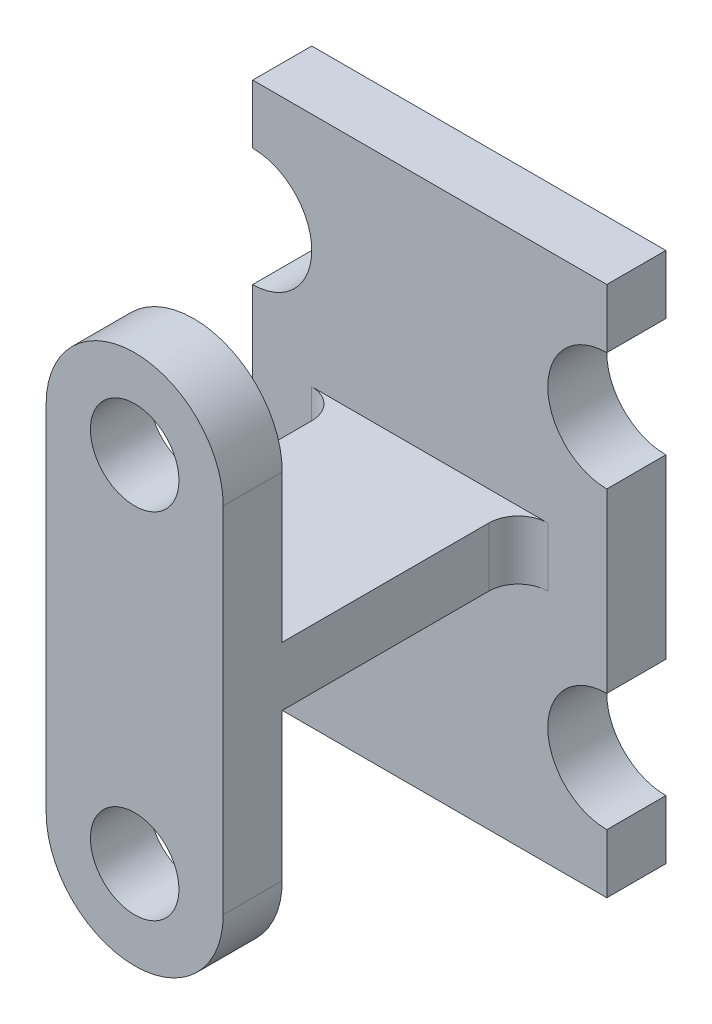
ISO-10303-21;
HEADER;
FILE_DESCRIPTION(('STEP AP214'),'2;1');
FILE_NAME('part.step','',(''),(''),'','','');
FILE_SCHEMA(('AUTOMOTIVE_DESIGN { 1 0 10303 214 1 1 1 1 }'));
ENDSEC;
DATA;
#1=APPLICATION_CONTEXT('core data for automotive mechanical design processes');
#2=APPLICATION_PROTOCOL_DEFINITION('international standard','automotive_design',2000,#1);
#3=PRODUCT_CONTEXT('',#1,'mechanical');
#4=PRODUCT('Part','Part','',(#3));
#5=PRODUCT_RELATED_PRODUCT_CATEGORY('part','',(#4));
#6=PRODUCT_DEFINITION_FORMATION('','',#4);
#7=PRODUCT_DEFINITION_CONTEXT('part definition',#1,'design');
#8=PRODUCT_DEFINITION('design','',#6,#7);
#9=PRODUCT_DEFINITION_SHAPE('','',#8);
#10=(LENGTH_UNIT() NAMED_UNIT(*) SI_UNIT(.MILLI.,.METRE.));
#11=(NAMED_UNIT(*) PLANE_ANGLE_UNIT() SI_UNIT($,.RADIAN.));
#12=(NAMED_UNIT(*) SI_UNIT($,.STERADIAN.) SOLID_ANGLE_UNIT());
#13=UNCERTAINTY_MEASURE_WITH_UNIT(LENGTH_MEASURE(1.E-05),#10,'distance_accuracy_value','');
#14=(GEOMETRIC_REPRESENTATION_CONTEXT(3) GLOBAL_UNCERTAINTY_ASSIGNED_CONTEXT((#13)) GLOBAL_UNIT_ASSIGNED_CONTEXT((#10,
#11,#12)) REPRESENTATION_CONTEXT('',''));
#15=CARTESIAN_POINT('',(0.,0.,0.));
#16=DIRECTION('',(0.,0.,1.));
#17=DIRECTION('',(1.,0.,0.));
#18=AXIS2_PLACEMENT_3D('',#15,#16,#17);
#19=CARTESIAN_POINT('',(3.,2.5,1.));
#20=DIRECTION('',(0.,0.,1.));
#21=DIRECTION('',(1.,0.,0.));
#22=AXIS2_PLACEMENT_3D('',#19,#20,#21);
#23=PLANE('',#22);
#24=DIRECTION('',(0.,1.,0.));
#25=VECTOR('',#24,1.);
#26=CARTESIAN_POINT('',(3.,4.5,1.));
#27=LINE('',#26,#25);
#28=CARTESIAN_POINT('',(3.,3.5,1.));
#29=VERTEX_POINT('',#28);
#30=CARTESIAN_POINT('',(3.,4.5,1.));
#31=VERTEX_POINT('',#30);
#32=EDGE_CURVE('E238',#29,#31,#27,.T.);
#33=ORIENTED_EDGE('',*,*,#32,.T.);
#34=DIRECTION('',(-1.,0.,0.));
#35=VECTOR('',#34,1.);
#36=CARTESIAN_POINT('',(-3.,4.5,1.));
#37=LINE('',#36,#35);
#38=CARTESIAN_POINT('',(-3.,4.5,1.));
#39=VERTEX_POINT('',#38);
#40=EDGE_CURVE('E244',#31,#39,#37,.T.);
#41=ORIENTED_EDGE('',*,*,#40,.T.);
#42=DIRECTION('',(0.,-1.,0.));
#43=VECTOR('',#42,1.);
#44=CARTESIAN_POINT('',(-3.,4.5,1.));
#45=LINE('',#44,#43);
#46=CARTESIAN_POINT('',(-3.,3.5,1.));
#47=VERTEX_POINT('',#46);
#48=EDGE_CURVE('E246',#39,#47,#45,.T.);
#49=ORIENTED_EDGE('',*,*,#48,.T.);
#50=CARTESIAN_POINT('',(-3.,2.5,1.));
#51=DIRECTION('',(0.,0.,-1.));
#52=DIRECTION('',(-1.,0.,0.));
#53=AXIS2_PLACEMENT_3D('',#50,#51,#52);
#54=CIRCLE('',#53,1.);
#55=CARTESIAN_POINT('',(-3.,1.5,1.));
#56=VERTEX_POINT('',#55);
#57=EDGE_CURVE('E248',#47,#56,#54,.T.);
#58=ORIENTED_EDGE('',*,*,#57,.T.);
#59=DIRECTION('',(0.,-1.,0.));
#60=VECTOR('',#59,1.);
#61=CARTESIAN_POINT('',(-3.,1.5,1.));
#62=LINE('',#61,#60);
#63=CARTESIAN_POINT('',(-3.,-1.5,1.));
#64=VERTEX_POINT('',#63);
#65=EDGE_CURVE('E249',#56,#64,#62,.T.);
#66=ORIENTED_EDGE('',*,*,#65,.T.);
#67=CARTESIAN_POINT('',(-3.,-2.5,1.));
#68=DIRECTION('',(0.,0.,-1.));
#69=DIRECTION('',(1.,0.,0.));
#70=AXIS2_PLACEMENT_3D('',#67,#68,#69);
#71=CIRCLE('',#70,1.);
#72=CARTESIAN_POINT('',(-3.,-3.5,1.));
#73=VERTEX_POINT('',#72);
#74=EDGE_CURVE('E252',#64,#73,#71,.T.);
#75=ORIENTED_EDGE('',*,*,#74,.T.);
#76=DIRECTION('',(0.,-1.,0.));
#77=VECTOR('',#76,1.);
#78=CARTESIAN_POINT('',(-3.,-4.5,1.));
#79=LINE('',#78,#77);
#80=CARTESIAN_POINT('',(-3.,-4.5,1.));
#81=VERTEX_POINT('',#80);
#82=EDGE_CURVE('E255',#73,#81,#79,.T.);
#83=ORIENTED_EDGE('',*,*,#82,.T.);
#84=DIRECTION('',(1.,0.,0.));
#85=VECTOR('',#84,1.);
#86=CARTESIAN_POINT('',(-3.,-4.5,1.));
#87=LINE('',#86,#85);
#88=CARTESIAN_POINT('',(3.,-4.5,1.));
#89=VERTEX_POINT('',#88);
#90=EDGE_CURVE('E258',#81,#89,#87,.T.);
#91=ORIENTED_EDGE('',*,*,#90,.T.);
#92=DIRECTION('',(0.,1.,0.));
#93=VECTOR('',#92,1.);
#94=CARTESIAN_POINT('',(3.,-4.5,1.));
#95=LINE('',#94,#93);
#96=CARTESIAN_POINT('',(3.,-3.5,1.));
#97=VERTEX_POINT('',#96);
#98=EDGE_CURVE('E256',#89,#97,#95,.T.);
#99=ORIENTED_EDGE('',*,*,#98,.T.);
#100=CARTESIAN_POINT('',(3.,-2.5,1.));
#101=DIRECTION('',(0.,0.,-1.));
#102=DIRECTION('',(-1.,0.,0.));
#103=AXIS2_PLACEMENT_3D('',#100,#101,#102);
#104=CIRCLE('',#103,1.);
#105=CARTESIAN_POINT('',(3.,-1.5,1.));
#106=VERTEX_POINT('',#105);
#107=EDGE_CURVE('E257',#97,#106,#104,.T.);
#108=ORIENTED_EDGE('',*,*,#107,.T.);
#109=DIRECTION('',(0.,1.,0.));
#110=VECTOR('',#109,1.);
#111=CARTESIAN_POINT('',(3.,1.5,1.));
#112=LINE('',#111,#110);
#113=CARTESIAN_POINT('',(3.,1.5,1.));
#114=VERTEX_POINT('',#113);
#115=EDGE_CURVE('E265',#106,#114,#112,.T.);
#116=ORIENTED_EDGE('',*,*,#115,.T.);
#117=CARTESIAN_POINT('',(3.,2.5,1.));
#118=DIRECTION('',(0.,0.,-1.));
#119=DIRECTION('',(1.,0.,0.));
#120=AXIS2_PLACEMENT_3D('',#117,#118,#119);
#121=CIRCLE('',#120,1.);
#122=EDGE_CURVE('E262',#114,#29,#121,.T.);
#123=ORIENTED_EDGE('',*,*,#122,.T.);
#124=EDGE_LOOP('',(#33,#41,#49,#58,#66,#75,#83,#91,#99,#108,#116,#123));
#125=FACE_BOUND('',#124,.T.);
#126=DIRECTION('',(-1.,0.,0.));
#127=VECTOR('',#126,1.);
#128=CARTESIAN_POINT('',(-1.5,0.5,1.));
#129=LINE('',#128,#127);
#130=CARTESIAN_POINT('',(2.,0.5,1.));
#131=VERTEX_POINT('',#130);
#132=CARTESIAN_POINT('',(-2.,0.5,1.));
#133=VERTEX_POINT('',#132);
#134=EDGE_CURVE('E213',#131,#133,#129,.T.);
#135=ORIENTED_EDGE('',*,*,#134,.F.);
#136=DIRECTION('',(0.,1.,0.));
#137=VECTOR('',#136,1.);
#138=CARTESIAN_POINT('',(2.,2.5,1.));
#139=LINE('',#138,#137);
#140=CARTESIAN_POINT('',(2.,-0.5,1.));
#141=VERTEX_POINT('',#140);
#142=EDGE_CURVE('E332',#131,#141,#139,.F.);
#143=ORIENTED_EDGE('',*,*,#142,.T.);
#144=DIRECTION('',(1.,0.,0.));
#145=VECTOR('',#144,1.);
#146=CARTESIAN_POINT('',(-1.5,-0.5,1.));
#147=LINE('',#146,#145);
#148=CARTESIAN_POINT('',(-2.,-0.5,1.));
#149=VERTEX_POINT('',#148);
#150=EDGE_CURVE('E214',#149,#141,#147,.T.);
#151=ORIENTED_EDGE('',*,*,#150,.F.);
#152=DIRECTION('',(0.,-1.,0.));
#153=VECTOR('',#152,1.);
#154=CARTESIAN_POINT('',(-2.,2.5,1.));
#155=LINE('',#154,#153);
#156=EDGE_CURVE('E327',#149,#133,#155,.F.);
#157=ORIENTED_EDGE('',*,*,#156,.T.);
#158=EDGE_LOOP('',(#135,#143,#151,#157));
#159=FACE_BOUND('',#158,.T.);
#160=ADVANCED_FACE('F39',(#125,#159),#23,.T.);
#161=CARTESIAN_POINT('',(3.,4.5,1.));
#162=DIRECTION('',(-1.,0.,0.));
#163=DIRECTION('',(0.,0.,1.));
#164=AXIS2_PLACEMENT_3D('',#161,#162,#163);
#165=PLANE('',#164);
#166=DIRECTION('',(0.,1.,0.));
#167=VECTOR('',#166,1.);
#168=CARTESIAN_POINT('',(3.,4.5,0.));
#169=LINE('',#168,#167);
#170=CARTESIAN_POINT('',(3.,3.5,0.));
#171=VERTEX_POINT('',#170);
#172=CARTESIAN_POINT('',(3.,4.5,0.));
#173=VERTEX_POINT('',#172);
#174=EDGE_CURVE('E239',#171,#173,#169,.T.);
#175=ORIENTED_EDGE('',*,*,#174,.T.);
#176=DIRECTION('',(0.,0.,-1.));
#177=VECTOR('',#176,1.);
#178=CARTESIAN_POINT('',(3.,4.5,1.));
#179=LINE('',#178,#177);
#180=EDGE_CURVE('E325',#31,#173,#179,.T.);
#181=ORIENTED_EDGE('',*,*,#180,.F.);
#182=ORIENTED_EDGE('',*,*,#32,.F.);
#183=DIRECTION('',(0.,0.,-1.));
#184=VECTOR('',#183,1.);
#185=CARTESIAN_POINT('',(3.,3.5,1.));
#186=LINE('',#185,#184);
#187=EDGE_CURVE('E266',#29,#171,#186,.T.);
#188=ORIENTED_EDGE('',*,*,#187,.T.);
#189=EDGE_LOOP('',(#175,#181,#182,#188));
#190=FACE_BOUND('',#189,.T.);
#191=ADVANCED_FACE('F388',(#190),#165,.F.);
#192=CARTESIAN_POINT('',(-3.,4.5,1.));
#193=DIRECTION('',(0.,-1.,0.));
#194=DIRECTION('',(0.,0.,-1.));
#195=AXIS2_PLACEMENT_3D('',#192,#193,#194);
#196=PLANE('',#195);
#197=DIRECTION('',(-1.,0.,0.));
#198=VECTOR('',#197,1.);
#199=CARTESIAN_POINT('',(-3.,4.5,0.));
#200=LINE('',#199,#198);
#201=CARTESIAN_POINT('',(-3.,4.5,0.));
#202=VERTEX_POINT('',#201);
#203=EDGE_CURVE('E267',#173,#202,#200,.T.);
#204=ORIENTED_EDGE('',*,*,#203,.T.);
#205=DIRECTION('',(0.,0.,-1.));
#206=VECTOR('',#205,1.);
#207=CARTESIAN_POINT('',(-3.,4.5,1.));
#208=LINE('',#207,#206);
#209=EDGE_CURVE('E317',#39,#202,#208,.T.);
#210=ORIENTED_EDGE('',*,*,#209,.F.);
#211=ORIENTED_EDGE('',*,*,#40,.F.);
#212=ORIENTED_EDGE('',*,*,#180,.T.);
#213=EDGE_LOOP('',(#204,#210,#211,#212));
#214=FACE_BOUND('',#213,.T.);
#215=ADVANCED_FACE('F398',(#214),#196,.F.);
#216=CARTESIAN_POINT('',(-3.,4.5,1.));
#217=DIRECTION('',(1.,0.,0.));
#218=DIRECTION('',(0.,0.,-1.));
#219=AXIS2_PLACEMENT_3D('',#216,#217,#218);
#220=PLANE('',#219);
#221=DIRECTION('',(0.,-1.,0.));
#222=VECTOR('',#221,1.);
#223=CARTESIAN_POINT('',(-3.,4.5,0.));
#224=LINE('',#223,#222);
#225=CARTESIAN_POINT('',(-3.,3.5,0.));
#226=VERTEX_POINT('',#225);
#227=EDGE_CURVE('E271',#202,#226,#224,.T.);
#228=ORIENTED_EDGE('',*,*,#227,.T.);
#229=DIRECTION('',(0.,0.,-1.));
#230=VECTOR('',#229,1.);
#231=CARTESIAN_POINT('',(-3.,3.5,1.));
#232=LINE('',#231,#230);
#233=EDGE_CURVE('E316',#47,#226,#232,.T.);
#234=ORIENTED_EDGE('',*,*,#233,.F.);
#235=ORIENTED_EDGE('',*,*,#48,.F.);
#236=ORIENTED_EDGE('',*,*,#209,.T.);
#237=EDGE_LOOP('',(#228,#234,#235,#236));
#238=FACE_BOUND('',#237,.T.);
#239=ADVANCED_FACE('F444',(#238),#220,.F.);
#240=CARTESIAN_POINT('',(-3.,2.5,1.));
#241=DIRECTION('',(0.,0.,-1.));
#242=DIRECTION('',(-1.,0.,0.));
#243=AXIS2_PLACEMENT_3D('',#240,#241,#242);
#244=CYLINDRICAL_SURFACE('',#243,1.);
#245=CARTESIAN_POINT('',(-3.,2.5,0.));
#246=DIRECTION('',(0.,0.,-1.));
#247=DIRECTION('',(-1.,0.,0.));
#248=AXIS2_PLACEMENT_3D('',#245,#246,#247);
#249=CIRCLE('',#248,1.);
#250=CARTESIAN_POINT('',(-3.,1.5,0.));
#251=VERTEX_POINT('',#250);
#252=EDGE_CURVE('E272',#226,#251,#249,.T.);
#253=ORIENTED_EDGE('',*,*,#252,.T.);
#254=DIRECTION('',(0.,0.,-1.));
#255=VECTOR('',#254,1.);
#256=CARTESIAN_POINT('',(-3.,1.5,1.));
#257=LINE('',#256,#255);
#258=EDGE_CURVE('E311',#56,#251,#257,.T.);
#259=ORIENTED_EDGE('',*,*,#258,.F.);
#260=ORIENTED_EDGE('',*,*,#57,.F.);
#261=ORIENTED_EDGE('',*,*,#233,.T.);
#262=EDGE_LOOP('',(#253,#259,#260,#261));
#263=FACE_BOUND('',#262,.T.);
#264=ADVANCED_FACE('F438',(#263),#244,.F.);
#265=CARTESIAN_POINT('',(-3.,1.5,1.));
#266=DIRECTION('',(1.,0.,0.));
#267=DIRECTION('',(0.,0.,-1.));
#268=AXIS2_PLACEMENT_3D('',#265,#266,#267);
#269=PLANE('',#268);
#270=DIRECTION('',(0.,-1.,0.));
#271=VECTOR('',#270,1.);
#272=CARTESIAN_POINT('',(-3.,1.5,0.));
#273=LINE('',#272,#271);
#274=CARTESIAN_POINT('',(-3.,-1.5,0.));
#275=VERTEX_POINT('',#274);
#276=EDGE_CURVE('E274',#251,#275,#273,.T.);
#277=ORIENTED_EDGE('',*,*,#276,.T.);
#278=DIRECTION('',(0.,0.,-1.));
#279=VECTOR('',#278,1.);
#280=CARTESIAN_POINT('',(-3.,-1.5,1.));
#281=LINE('',#280,#279);
#282=EDGE_CURVE('E309',#64,#275,#281,.T.);
#283=ORIENTED_EDGE('',*,*,#282,.F.);
#284=ORIENTED_EDGE('',*,*,#65,.F.);
#285=ORIENTED_EDGE('',*,*,#258,.T.);
#286=EDGE_LOOP('',(#277,#283,#284,#285));
#287=FACE_BOUND('',#286,.T.);
#288=ADVANCED_FACE('F434',(#287),#269,.F.);
#289=CARTESIAN_POINT('',(-3.,-2.5,1.));
#290=DIRECTION('',(0.,0.,-1.));
#291=DIRECTION('',(-1.,0.,0.));
#292=AXIS2_PLACEMENT_3D('',#289,#290,#291);
#293=CYLINDRICAL_SURFACE('',#292,1.);
#294=CARTESIAN_POINT('',(-3.,-2.5,0.));
#295=DIRECTION('',(0.,0.,-1.));
#296=DIRECTION('',(1.,0.,0.));
#297=AXIS2_PLACEMENT_3D('',#294,#295,#296);
#298=CIRCLE('',#297,1.);
#299=CARTESIAN_POINT('',(-3.,-3.5,0.));
#300=VERTEX_POINT('',#299);
#301=EDGE_CURVE('E280',#275,#300,#298,.T.);
#302=ORIENTED_EDGE('',*,*,#301,.T.);
#303=DIRECTION('',(0.,0.,-1.));
#304=VECTOR('',#303,1.);
#305=CARTESIAN_POINT('',(-3.,-3.5,1.));
#306=LINE('',#305,#304);
#307=EDGE_CURVE('E307',#73,#300,#306,.T.);
#308=ORIENTED_EDGE('',*,*,#307,.F.);
#309=ORIENTED_EDGE('',*,*,#74,.F.);
#310=ORIENTED_EDGE('',*,*,#282,.T.);
#311=EDGE_LOOP('',(#302,#308,#309,#310));
#312=FACE_BOUND('',#311,.T.);
#313=ADVANCED_FACE('F431',(#312),#293,.F.);
#314=CARTESIAN_POINT('',(-3.,-4.5,1.));
#315=DIRECTION('',(1.,0.,0.));
#316=DIRECTION('',(0.,0.,-1.));
#317=AXIS2_PLACEMENT_3D('',#314,#315,#316);
#318=PLANE('',#317);
#319=DIRECTION('',(0.,-1.,0.));
#320=VECTOR('',#319,1.);
#321=CARTESIAN_POINT('',(-3.,-4.5,0.));
#322=LINE('',#321,#320);
#323=CARTESIAN_POINT('',(-3.,-4.5,0.));
#324=VERTEX_POINT('',#323);
#325=EDGE_CURVE('E276',#300,#324,#322,.T.);
#326=ORIENTED_EDGE('',*,*,#325,.T.);
#327=DIRECTION('',(0.,0.,-1.));
#328=VECTOR('',#327,1.);
#329=CARTESIAN_POINT('',(-3.,-4.5,1.));
#330=LINE('',#329,#328);
#331=EDGE_CURVE('E302',#81,#324,#330,.T.);
#332=ORIENTED_EDGE('',*,*,#331,.F.);
#333=ORIENTED_EDGE('',*,*,#82,.F.);
#334=ORIENTED_EDGE('',*,*,#307,.T.);
#335=EDGE_LOOP('',(#326,#332,#333,#334));
#336=FACE_BOUND('',#335,.T.);
#337=ADVANCED_FACE('F430',(#336),#318,.F.);
#338=CARTESIAN_POINT('',(-3.,-4.5,1.));
#339=DIRECTION('',(0.,1.,0.));
#340=DIRECTION('',(0.,0.,1.));
#341=AXIS2_PLACEMENT_3D('',#338,#339,#340);
#342=PLANE('',#341);
#343=DIRECTION('',(1.,0.,0.));
#344=VECTOR('',#343,1.);
#345=CARTESIAN_POINT('',(-3.,-4.5,0.));
#346=LINE('',#345,#344);
#347=CARTESIAN_POINT('',(3.,-4.5,0.));
#348=VERTEX_POINT('',#347);
#349=EDGE_CURVE('E281',#324,#348,#346,.T.);
#350=ORIENTED_EDGE('',*,*,#349,.T.);
#351=DIRECTION('',(0.,0.,-1.));
#352=VECTOR('',#351,1.);
#353=CARTESIAN_POINT('',(3.,-4.5,1.));
#354=LINE('',#353,#352);
#355=EDGE_CURVE('E301',#89,#348,#354,.T.);
#356=ORIENTED_EDGE('',*,*,#355,.F.);
#357=ORIENTED_EDGE('',*,*,#90,.F.);
#358=ORIENTED_EDGE('',*,*,#331,.T.);
#359=EDGE_LOOP('',(#350,#356,#357,#358));
#360=FACE_BOUND('',#359,.T.);
#361=ADVANCED_FACE('F421',(#360),#342,.F.);
#362=CARTESIAN_POINT('',(3.,-4.5,1.));
#363=DIRECTION('',(-1.,0.,0.));
#364=DIRECTION('',(0.,0.,1.));
#365=AXIS2_PLACEMENT_3D('',#362,#363,#364);
#366=PLANE('',#365);
#367=DIRECTION('',(0.,1.,0.));
#368=VECTOR('',#367,1.);
#369=CARTESIAN_POINT('',(3.,-4.5,0.));
#370=LINE('',#369,#368);
#371=CARTESIAN_POINT('',(3.,-3.5,0.));
#372=VERTEX_POINT('',#371);
#373=EDGE_CURVE('E284',#348,#372,#370,.T.);
#374=ORIENTED_EDGE('',*,*,#373,.T.);
#375=DIRECTION('',(0.,0.,-1.));
#376=VECTOR('',#375,1.);
#377=CARTESIAN_POINT('',(3.,-3.5,1.));
#378=LINE('',#377,#376);
#379=EDGE_CURVE('E299',#97,#372,#378,.T.);
#380=ORIENTED_EDGE('',*,*,#379,.F.);
#381=ORIENTED_EDGE('',*,*,#98,.F.);
#382=ORIENTED_EDGE('',*,*,#355,.T.);
#383=EDGE_LOOP('',(#374,#380,#381,#382));
#384=FACE_BOUND('',#383,.T.);
#385=ADVANCED_FACE('F420',(#384),#366,.F.);
#386=CARTESIAN_POINT('',(3.,-2.5,1.));
#387=DIRECTION('',(0.,0.,-1.));
#388=DIRECTION('',(-1.,0.,0.));
#389=AXIS2_PLACEMENT_3D('',#386,#387,#388);
#390=CYLINDRICAL_SURFACE('',#389,1.);
#391=CARTESIAN_POINT('',(3.,-2.5,0.));
#392=DIRECTION('',(0.,0.,-1.));
#393=DIRECTION('',(-1.,0.,0.));
#394=AXIS2_PLACEMENT_3D('',#391,#392,#393);
#395=CIRCLE('',#394,1.);
#396=CARTESIAN_POINT('',(3.,-1.5,0.));
#397=VERTEX_POINT('',#396);
#398=EDGE_CURVE('E285',#372,#397,#395,.T.);
#399=ORIENTED_EDGE('',*,*,#398,.T.);
#400=DIRECTION('',(0.,0.,-1.));
#401=VECTOR('',#400,1.);
#402=CARTESIAN_POINT('',(3.,-1.5,1.));
#403=LINE('',#402,#401);
#404=EDGE_CURVE('E293',#106,#397,#403,.T.);
#405=ORIENTED_EDGE('',*,*,#404,.F.);
#406=ORIENTED_EDGE('',*,*,#107,.F.);
#407=ORIENTED_EDGE('',*,*,#379,.T.);
#408=EDGE_LOOP('',(#399,#405,#406,#407));
#409=FACE_BOUND('',#408,.T.);
#410=ADVANCED_FACE('F414',(#409),#390,.F.);
#411=CARTESIAN_POINT('',(3.,1.5,1.));
#412=DIRECTION('',(-1.,0.,0.));
#413=DIRECTION('',(0.,0.,1.));
#414=AXIS2_PLACEMENT_3D('',#411,#412,#413);
#415=PLANE('',#414);
#416=DIRECTION('',(0.,1.,0.));
#417=VECTOR('',#416,1.);
#418=CARTESIAN_POINT('',(3.,1.5,0.));
#419=LINE('',#418,#417);
#420=CARTESIAN_POINT('',(3.,1.5,0.));
#421=VERTEX_POINT('',#420);
#422=EDGE_CURVE('E290',#397,#421,#419,.T.);
#423=ORIENTED_EDGE('',*,*,#422,.T.);
#424=DIRECTION('',(0.,0.,-1.));
#425=VECTOR('',#424,1.);
#426=CARTESIAN_POINT('',(3.,1.5,1.));
#427=LINE('',#426,#425);
#428=EDGE_CURVE('E295',#114,#421,#427,.T.);
#429=ORIENTED_EDGE('',*,*,#428,.F.);
#430=ORIENTED_EDGE('',*,*,#115,.F.);
#431=ORIENTED_EDGE('',*,*,#404,.T.);
#432=EDGE_LOOP('',(#423,#429,#430,#431));
#433=FACE_BOUND('',#432,.T.);
#434=ADVANCED_FACE('F411',(#433),#415,.F.);
#435=CARTESIAN_POINT('',(3.,2.5,1.));
#436=DIRECTION('',(0.,0.,-1.));
#437=DIRECTION('',(-1.,0.,0.));
#438=AXIS2_PLACEMENT_3D('',#435,#436,#437);
#439=CYLINDRICAL_SURFACE('',#438,1.);
#440=CARTESIAN_POINT('',(3.,2.5,0.));
#441=DIRECTION('',(0.,0.,-1.));
#442=DIRECTION('',(1.,0.,0.));
#443=AXIS2_PLACEMENT_3D('',#440,#441,#442);
#444=CIRCLE('',#443,1.);
#445=EDGE_CURVE('E243',#421,#171,#444,.T.);
#446=ORIENTED_EDGE('',*,*,#445,.T.);
#447=ORIENTED_EDGE('',*,*,#187,.F.);
#448=ORIENTED_EDGE('',*,*,#122,.F.);
#449=ORIENTED_EDGE('',*,*,#428,.T.);
#450=EDGE_LOOP('',(#446,#447,#448,#449));
#451=FACE_BOUND('',#450,.T.);
#452=ADVANCED_FACE('F407',(#451),#439,.F.);
#453=CARTESIAN_POINT('',(3.,2.5,0.));
#454=DIRECTION('',(0.,0.,1.));
#455=DIRECTION('',(1.,0.,0.));
#456=AXIS2_PLACEMENT_3D('',#453,#454,#455);
#457=PLANE('',#456);
#458=ORIENTED_EDGE('',*,*,#174,.F.);
#459=ORIENTED_EDGE('',*,*,#445,.F.);
#460=ORIENTED_EDGE('',*,*,#422,.F.);
#461=ORIENTED_EDGE('',*,*,#398,.F.);
#462=ORIENTED_EDGE('',*,*,#373,.F.);
#463=ORIENTED_EDGE('',*,*,#349,.F.);
#464=ORIENTED_EDGE('',*,*,#325,.F.);
#465=ORIENTED_EDGE('',*,*,#301,.F.);
#466=ORIENTED_EDGE('',*,*,#276,.F.);
#467=ORIENTED_EDGE('',*,*,#252,.F.);
#468=ORIENTED_EDGE('',*,*,#227,.F.);
#469=ORIENTED_EDGE('',*,*,#203,.F.);
#470=EDGE_LOOP('',(#458,#459,#460,#461,#462,#463,#464,#465,#466,#467,#468,#469));
#471=FACE_BOUND('',#470,.T.);
#472=ADVANCED_FACE('F404',(#471),#457,.F.);
#473=CARTESIAN_POINT('',(1.5,0.5,5.));
#474=DIRECTION('',(-1.,0.,0.));
#475=DIRECTION('',(0.,-1.,0.));
#476=AXIS2_PLACEMENT_3D('',#473,#474,#475);
#477=PLANE('',#476);
#478=DIRECTION('',(0.,0.,-1.));
#479=VECTOR('',#478,1.);
#480=CARTESIAN_POINT('',(1.5,-0.5,5.));
#481=LINE('',#480,#479);
#482=CARTESIAN_POINT('',(1.5,-0.5,5.));
#483=VERTEX_POINT('',#482);
#484=CARTESIAN_POINT('',(1.5,-0.5,1.5));
#485=VERTEX_POINT('',#484);
#486=EDGE_CURVE('E226',#483,#485,#481,.T.);
#487=ORIENTED_EDGE('',*,*,#486,.T.);
#488=DIRECTION('',(0.,1.,0.));
#489=VECTOR('',#488,1.);
#490=CARTESIAN_POINT('',(1.5,0.5,1.5));
#491=LINE('',#490,#489);
#492=CARTESIAN_POINT('',(1.5,0.5,1.5));
#493=VERTEX_POINT('',#492);
#494=EDGE_CURVE('E324',#485,#493,#491,.T.);
#495=ORIENTED_EDGE('',*,*,#494,.T.);
#496=DIRECTION('',(0.,0.,-1.));
#497=VECTOR('',#496,1.);
#498=CARTESIAN_POINT('',(1.5,0.5,5.));
#499=LINE('',#498,#497);
#500=CARTESIAN_POINT('',(1.5,0.5,5.));
#501=VERTEX_POINT('',#500);
#502=EDGE_CURVE('E237',#501,#493,#499,.T.);
#503=ORIENTED_EDGE('',*,*,#502,.F.);
#504=DIRECTION('',(0.,1.,0.));
#505=VECTOR('',#504,1.);
#506=CARTESIAN_POINT('',(1.5,3.,5.));
#507=LINE('',#506,#505);
#508=CARTESIAN_POINT('',(1.5,3.,5.));
#509=VERTEX_POINT('',#508);
#510=EDGE_CURVE('E358',#501,#509,#507,.T.);
#511=ORIENTED_EDGE('',*,*,#510,.T.);
#512=DIRECTION('',(0.,0.,-1.));
#513=VECTOR('',#512,1.);
#514=CARTESIAN_POINT('',(1.5,3.,6.));
#515=LINE('',#514,#513);
#516=CARTESIAN_POINT('',(1.5,3.,6.));
#517=VERTEX_POINT('',#516);
#518=EDGE_CURVE('E365',#517,#509,#515,.T.);
#519=ORIENTED_EDGE('',*,*,#518,.F.);
#520=DIRECTION('',(0.,1.,0.));
#521=VECTOR('',#520,1.);
#522=CARTESIAN_POINT('',(1.5,3.,6.));
#523=LINE('',#522,#521);
#524=CARTESIAN_POINT('',(1.5,-3.,6.));
#525=VERTEX_POINT('',#524);
#526=EDGE_CURVE('E204',#525,#517,#523,.T.);
#527=ORIENTED_EDGE('',*,*,#526,.F.);
#528=DIRECTION('',(0.,0.,-1.));
#529=VECTOR('',#528,1.);
#530=CARTESIAN_POINT('',(1.5,-3.,6.));
#531=LINE('',#530,#529);
#532=CARTESIAN_POINT('',(1.5,-3.,5.));
#533=VERTEX_POINT('',#532);
#534=EDGE_CURVE('E220',#525,#533,#531,.T.);
#535=ORIENTED_EDGE('',*,*,#534,.T.);
#536=EDGE_CURVE('E208',#533,#483,#507,.T.);
#537=ORIENTED_EDGE('',*,*,#536,.T.);
#538=EDGE_LOOP('',(#487,#495,#503,#511,#519,#527,#535,#537));
#539=FACE_BOUND('',#538,.T.);
#540=ADVANCED_FACE('F351',(#539),#477,.F.);
#541=CARTESIAN_POINT('',(-1.5,0.5,5.));
#542=DIRECTION('',(0.,-1.,0.));
#543=DIRECTION('',(0.,0.,-1.));
#544=AXIS2_PLACEMENT_3D('',#541,#542,#543);
#545=PLANE('',#544);
#546=ORIENTED_EDGE('',*,*,#134,.T.);
#547=CARTESIAN_POINT('',(-2.,0.5,1.5));
#548=DIRECTION('',(0.,-1.,0.));
#549=DIRECTION('',(0.,0.,-1.));
#550=AXIS2_PLACEMENT_3D('',#547,#548,#549);
#551=CIRCLE('',#550,0.5);
#552=CARTESIAN_POINT('',(-1.5,0.5,1.5));
#553=VERTEX_POINT('',#552);
#554=EDGE_CURVE('E11',#133,#553,#551,.T.);
#555=ORIENTED_EDGE('',*,*,#554,.T.);
#556=DIRECTION('',(0.,0.,-1.));
#557=VECTOR('',#556,1.);
#558=CARTESIAN_POINT('',(-1.5,0.5,5.));
#559=LINE('',#558,#557);
#560=CARTESIAN_POINT('',(-1.5,0.5,5.));
#561=VERTEX_POINT('',#560);
#562=EDGE_CURVE('E232',#561,#553,#559,.T.);
#563=ORIENTED_EDGE('',*,*,#562,.F.);
#564=DIRECTION('',(-1.,0.,0.));
#565=VECTOR('',#564,1.);
#566=CARTESIAN_POINT('',(-1.5,0.5,5.));
#567=LINE('',#566,#565);
#568=EDGE_CURVE('E222',#501,#561,#567,.T.);
#569=ORIENTED_EDGE('',*,*,#568,.F.);
#570=ORIENTED_EDGE('',*,*,#502,.T.);
#571=CARTESIAN_POINT('',(2.,0.5,1.5));
#572=DIRECTION('',(0.,-1.,0.));
#573=DIRECTION('',(0.,0.,-1.));
#574=AXIS2_PLACEMENT_3D('',#571,#572,#573);
#575=CIRCLE('',#574,0.5);
#576=EDGE_CURVE('E336',#493,#131,#575,.T.);
#577=ORIENTED_EDGE('',*,*,#576,.T.);
#578=EDGE_LOOP('',(#546,#555,#563,#569,#570,#577));
#579=FACE_BOUND('',#578,.T.);
#580=ADVANCED_FACE('F486',(#579),#545,.F.);
#581=CARTESIAN_POINT('',(-1.5,0.5,5.));
#582=DIRECTION('',(1.,0.,0.));
#583=DIRECTION('',(0.,1.,0.));
#584=AXIS2_PLACEMENT_3D('',#581,#582,#583);
#585=PLANE('',#584);
#586=ORIENTED_EDGE('',*,*,#562,.T.);
#587=DIRECTION('',(0.,-1.,0.));
#588=VECTOR('',#587,1.);
#589=CARTESIAN_POINT('',(-1.5,0.5,1.5));
#590=LINE('',#589,#588);
#591=CARTESIAN_POINT('',(-1.5,-0.5,1.5));
#592=VERTEX_POINT('',#591);
#593=EDGE_CURVE('E331',#553,#592,#590,.T.);
#594=ORIENTED_EDGE('',*,*,#593,.T.);
#595=DIRECTION('',(0.,0.,-1.));
#596=VECTOR('',#595,1.);
#597=CARTESIAN_POINT('',(-1.5,-0.5,5.));
#598=LINE('',#597,#596);
#599=CARTESIAN_POINT('',(-1.5,-0.5,5.));
#600=VERTEX_POINT('',#599);
#601=EDGE_CURVE('E231',#600,#592,#598,.T.);
#602=ORIENTED_EDGE('',*,*,#601,.F.);
#603=DIRECTION('',(0.,-1.,0.));
#604=VECTOR('',#603,1.);
#605=CARTESIAN_POINT('',(-1.5,3.,5.));
#606=LINE('',#605,#604);
#607=CARTESIAN_POINT('',(-1.5,-3.,5.));
#608=VERTEX_POINT('',#607);
#609=EDGE_CURVE('E366',#600,#608,#606,.T.);
#610=ORIENTED_EDGE('',*,*,#609,.T.);
#611=DIRECTION('',(0.,0.,-1.));
#612=VECTOR('',#611,1.);
#613=CARTESIAN_POINT('',(-1.5,-3.,6.));
#614=LINE('',#613,#612);
#615=CARTESIAN_POINT('',(-1.5,-3.,6.));
#616=VERTEX_POINT('',#615);
#617=EDGE_CURVE('E194',#616,#608,#614,.T.);
#618=ORIENTED_EDGE('',*,*,#617,.F.);
#619=DIRECTION('',(0.,-1.,0.));
#620=VECTOR('',#619,1.);
#621=CARTESIAN_POINT('',(-1.5,3.,6.));
#622=LINE('',#621,#620);
#623=CARTESIAN_POINT('',(-1.5,3.,6.));
#624=VERTEX_POINT('',#623);
#625=EDGE_CURVE('E187',#624,#616,#622,.T.);
#626=ORIENTED_EDGE('',*,*,#625,.F.);
#627=DIRECTION('',(0.,0.,-1.));
#628=VECTOR('',#627,1.);
#629=CARTESIAN_POINT('',(-1.5,3.,6.));
#630=LINE('',#629,#628);
#631=CARTESIAN_POINT('',(-1.5,3.,5.));
#632=VERTEX_POINT('',#631);
#633=EDGE_CURVE('E195',#624,#632,#630,.T.);
#634=ORIENTED_EDGE('',*,*,#633,.T.);
#635=EDGE_CURVE('E367',#632,#561,#606,.T.);
#636=ORIENTED_EDGE('',*,*,#635,.T.);
#637=EDGE_LOOP('',(#586,#594,#602,#610,#618,#626,#634,#636));
#638=FACE_BOUND('',#637,.T.);
#639=ADVANCED_FACE('F188',(#638),#585,.F.);
#640=CARTESIAN_POINT('',(-1.5,-0.5,5.));
#641=DIRECTION('',(0.,1.,0.));
#642=DIRECTION('',(0.,0.,1.));
#643=AXIS2_PLACEMENT_3D('',#640,#641,#642);
#644=PLANE('',#643);
#645=ORIENTED_EDGE('',*,*,#150,.T.);
#646=CARTESIAN_POINT('',(2.,-0.5,1.5));
#647=DIRECTION('',(0.,1.,0.));
#648=DIRECTION('',(0.,0.,1.));
#649=AXIS2_PLACEMENT_3D('',#646,#647,#648);
#650=CIRCLE('',#649,0.5);
#651=EDGE_CURVE('E338',#141,#485,#650,.T.);
#652=ORIENTED_EDGE('',*,*,#651,.T.);
#653=ORIENTED_EDGE('',*,*,#486,.F.);
#654=DIRECTION('',(1.,0.,0.));
#655=VECTOR('',#654,1.);
#656=CARTESIAN_POINT('',(-1.5,-0.5,5.));
#657=LINE('',#656,#655);
#658=EDGE_CURVE('E221',#600,#483,#657,.T.);
#659=ORIENTED_EDGE('',*,*,#658,.F.);
#660=ORIENTED_EDGE('',*,*,#601,.T.);
#661=CARTESIAN_POINT('',(-2.,-0.5,1.5));
#662=DIRECTION('',(0.,1.,0.));
#663=DIRECTION('',(0.,0.,1.));
#664=AXIS2_PLACEMENT_3D('',#661,#662,#663);
#665=CIRCLE('',#664,0.5);
#666=EDGE_CURVE('E50',#592,#149,#665,.T.);
#667=ORIENTED_EDGE('',*,*,#666,.T.);
#668=EDGE_LOOP('',(#645,#652,#653,#659,#660,#667));
#669=FACE_BOUND('',#668,.T.);
#670=ADVANCED_FACE('F341',(#669),#644,.F.);
#671=CARTESIAN_POINT('',(0.,3.,5.));
#672=DIRECTION('',(0.,0.,1.));
#673=DIRECTION('',(1.,0.,0.));
#674=AXIS2_PLACEMENT_3D('',#671,#672,#673);
#675=PLANE('',#674);
#676=CARTESIAN_POINT('',(0.,3.,5.));
#677=DIRECTION('',(0.,0.,1.));
#678=DIRECTION('',(1.,0.,0.));
#679=AXIS2_PLACEMENT_3D('',#676,#677,#678);
#680=CIRCLE('',#679,0.75);
#681=CARTESIAN_POINT('',(0.750000000000001,3.,5.));
#682=VERTEX_POINT('',#681);
#683=EDGE_CURVE('E369',#682,#682,#680,.T.);
#684=ORIENTED_EDGE('',*,*,#683,.T.);
#685=EDGE_LOOP('',(#684));
#686=FACE_BOUND('',#685,.T.);
#687=ORIENTED_EDGE('',*,*,#510,.F.);
#688=ORIENTED_EDGE('',*,*,#568,.T.);
#689=ORIENTED_EDGE('',*,*,#635,.F.);
#690=CARTESIAN_POINT('',(0.,3.,5.));
#691=DIRECTION('',(0.,0.,1.));
#692=DIRECTION('',(1.,0.,0.));
#693=AXIS2_PLACEMENT_3D('',#690,#691,#692);
#694=CIRCLE('',#693,1.5);
#695=EDGE_CURVE('E215',#509,#632,#694,.T.);
#696=ORIENTED_EDGE('',*,*,#695,.F.);
#697=EDGE_LOOP('',(#687,#688,#689,#696));
#698=FACE_BOUND('',#697,.T.);
#699=ADVANCED_FACE('F376',(#686,#698),#675,.F.);
#700=CARTESIAN_POINT('',(0.,-3.,5.));
#701=DIRECTION('',(0.,0.,1.));
#702=DIRECTION('',(1.,0.,0.));
#703=AXIS2_PLACEMENT_3D('',#700,#701,#702);
#704=CIRCLE('',#703,0.75);
#705=CARTESIAN_POINT('',(0.75,-3.,5.));
#706=VERTEX_POINT('',#705);
#707=EDGE_CURVE('E476',#706,#706,#704,.T.);
#708=ORIENTED_EDGE('',*,*,#707,.T.);
#709=EDGE_LOOP('',(#708));
#710=FACE_BOUND('',#709,.T.);
#711=ORIENTED_EDGE('',*,*,#609,.F.);
#712=ORIENTED_EDGE('',*,*,#658,.T.);
#713=ORIENTED_EDGE('',*,*,#536,.F.);
#714=CARTESIAN_POINT('',(0.,-3.,5.));
#715=DIRECTION('',(0.,0.,1.));
#716=DIRECTION('',(1.,0.,0.));
#717=AXIS2_PLACEMENT_3D('',#714,#715,#716);
#718=CIRCLE('',#717,1.5);
#719=EDGE_CURVE('E359',#608,#533,#718,.T.);
#720=ORIENTED_EDGE('',*,*,#719,.F.);
#721=EDGE_LOOP('',(#711,#712,#713,#720));
#722=FACE_BOUND('',#721,.T.);
#723=ADVANCED_FACE('F372',(#710,#722),#675,.F.);
#724=CARTESIAN_POINT('',(0.,3.,6.));
#725=DIRECTION('',(0.,0.,-1.));
#726=DIRECTION('',(-1.,0.,0.));
#727=AXIS2_PLACEMENT_3D('',#724,#725,#726);
#728=CYLINDRICAL_SURFACE('',#727,1.5);
#729=ORIENTED_EDGE('',*,*,#695,.T.);
#730=ORIENTED_EDGE('',*,*,#633,.F.);
#731=CARTESIAN_POINT('',(0.,3.,6.));
#732=DIRECTION('',(0.,0.,1.));
#733=DIRECTION('',(1.,0.,0.));
#734=AXIS2_PLACEMENT_3D('',#731,#732,#733);
#735=CIRCLE('',#734,1.5);
#736=EDGE_CURVE('E200',#517,#624,#735,.T.);
#737=ORIENTED_EDGE('',*,*,#736,.F.);
#738=ORIENTED_EDGE('',*,*,#518,.T.);
#739=EDGE_LOOP('',(#729,#730,#737,#738));
#740=FACE_BOUND('',#739,.T.);
#741=ADVANCED_FACE('F209',(#740),#728,.T.);
#742=CARTESIAN_POINT('',(0.,-3.,6.));
#743=DIRECTION('',(0.,0.,-1.));
#744=DIRECTION('',(-1.,0.,0.));
#745=AXIS2_PLACEMENT_3D('',#742,#743,#744);
#746=CYLINDRICAL_SURFACE('',#745,1.5);
#747=ORIENTED_EDGE('',*,*,#719,.T.);
#748=ORIENTED_EDGE('',*,*,#534,.F.);
#749=CARTESIAN_POINT('',(0.,-3.,6.));
#750=DIRECTION('',(0.,0.,1.));
#751=DIRECTION('',(1.,0.,0.));
#752=AXIS2_PLACEMENT_3D('',#749,#750,#751);
#753=CIRCLE('',#752,1.5);
#754=EDGE_CURVE('E196',#616,#525,#753,.T.);
#755=ORIENTED_EDGE('',*,*,#754,.F.);
#756=ORIENTED_EDGE('',*,*,#617,.T.);
#757=EDGE_LOOP('',(#747,#748,#755,#756));
#758=FACE_BOUND('',#757,.T.);
#759=ADVANCED_FACE('F373',(#758),#746,.T.);
#760=CARTESIAN_POINT('',(0.,3.,6.));
#761=DIRECTION('',(0.,0.,1.));
#762=DIRECTION('',(1.,0.,0.));
#763=AXIS2_PLACEMENT_3D('',#760,#761,#762);
#764=PLANE('',#763);
#765=CARTESIAN_POINT('',(0.,3.,6.));
#766=DIRECTION('',(0.,0.,1.));
#767=DIRECTION('',(1.,0.,0.));
#768=AXIS2_PLACEMENT_3D('',#765,#766,#767);
#769=CIRCLE('',#768,0.75);
#770=CARTESIAN_POINT('',(0.750000000000001,3.,6.));
#771=VERTEX_POINT('',#770);
#772=EDGE_CURVE('E471',#771,#771,#769,.T.);
#773=ORIENTED_EDGE('',*,*,#772,.F.);
#774=EDGE_LOOP('',(#773));
#775=FACE_BOUND('',#774,.T.);
#776=CARTESIAN_POINT('',(0.,-3.,6.));
#777=DIRECTION('',(0.,0.,1.));
#778=DIRECTION('',(1.,0.,0.));
#779=AXIS2_PLACEMENT_3D('',#776,#777,#778);
#780=CIRCLE('',#779,0.75);
#781=CARTESIAN_POINT('',(0.75,-3.,6.));
#782=VERTEX_POINT('',#781);
#783=EDGE_CURVE('E478',#782,#782,#780,.T.);
#784=ORIENTED_EDGE('',*,*,#783,.F.);
#785=EDGE_LOOP('',(#784));
#786=FACE_BOUND('',#785,.T.);
#787=ORIENTED_EDGE('',*,*,#736,.T.);
#788=ORIENTED_EDGE('',*,*,#625,.T.);
#789=ORIENTED_EDGE('',*,*,#754,.T.);
#790=ORIENTED_EDGE('',*,*,#526,.T.);
#791=EDGE_LOOP('',(#787,#788,#789,#790));
#792=FACE_BOUND('',#791,.T.);
#793=ADVANCED_FACE('F205',(#775,#786,#792),#764,.T.);
#794=CARTESIAN_POINT('',(0.,-3.,5.));
#795=DIRECTION('',(0.,0.,1.));
#796=DIRECTION('',(1.,0.,0.));
#797=AXIS2_PLACEMENT_3D('',#794,#795,#796);
#798=CYLINDRICAL_SURFACE('',#797,0.75);
#799=ORIENTED_EDGE('',*,*,#707,.F.);
#800=EDGE_LOOP('',(#799));
#801=FACE_BOUND('',#800,.T.);
#802=ORIENTED_EDGE('',*,*,#783,.T.);
#803=EDGE_LOOP('',(#802));
#804=FACE_BOUND('',#803,.T.);
#805=ADVANCED_FACE('F457',(#801,#804),#798,.F.);
#806=CARTESIAN_POINT('',(0.,3.,5.));
#807=DIRECTION('',(0.,0.,1.));
#808=DIRECTION('',(1.,0.,0.));
#809=AXIS2_PLACEMENT_3D('',#806,#807,#808);
#810=CYLINDRICAL_SURFACE('',#809,0.75);
#811=ORIENTED_EDGE('',*,*,#683,.F.);
#812=EDGE_LOOP('',(#811));
#813=FACE_BOUND('',#812,.T.);
#814=ORIENTED_EDGE('',*,*,#772,.T.);
#815=EDGE_LOOP('',(#814));
#816=FACE_BOUND('',#815,.T.);
#817=ADVANCED_FACE('F451',(#813,#816),#810,.F.);
#818=CARTESIAN_POINT('',(2.,0.5,1.5));
#819=DIRECTION('',(0.,1.,0.));
#820=DIRECTION('',(-1.,0.,0.));
#821=AXIS2_PLACEMENT_3D('',#818,#819,#820);
#822=CYLINDRICAL_SURFACE('',#821,0.5);
#823=ORIENTED_EDGE('',*,*,#651,.F.);
#824=ORIENTED_EDGE('',*,*,#142,.F.);
#825=ORIENTED_EDGE('',*,*,#576,.F.);
#826=ORIENTED_EDGE('',*,*,#494,.F.);
#827=EDGE_LOOP('',(#823,#824,#825,#826));
#828=FACE_BOUND('',#827,.T.);
#829=ADVANCED_FACE('F346',(#828),#822,.F.);
#830=CARTESIAN_POINT('',(-2.,0.5,1.5));
#831=DIRECTION('',(0.,-1.,0.));
#832=DIRECTION('',(1.,0.,0.));
#833=AXIS2_PLACEMENT_3D('',#830,#831,#832);
#834=CYLINDRICAL_SURFACE('',#833,0.5);
#835=ORIENTED_EDGE('',*,*,#554,.F.);
#836=ORIENTED_EDGE('',*,*,#156,.F.);
#837=ORIENTED_EDGE('',*,*,#666,.F.);
#838=ORIENTED_EDGE('',*,*,#593,.F.);
#839=EDGE_LOOP('',(#835,#836,#837,#838));
#840=FACE_BOUND('',#839,.T.);
#841=ADVANCED_FACE('F41',(#840),#834,.F.);
#842=CLOSED_SHELL('',(#160,#191,#215,#239,#264,#288,#313,#337,#361,#385,#410,#434,#452,#472,
#540,#580,#639,#670,#699,#723,#741,#759,#793,#805,#817,#829,#841));
#843=MANIFOLD_SOLID_BREP('B2',#842);
#844=ADVANCED_BREP_SHAPE_REPRESENTATION('',(#18,#843),#14);
#845=SHAPE_DEFINITION_REPRESENTATION(#9,#844);
ENDSEC;
END-ISO-10303-21;
